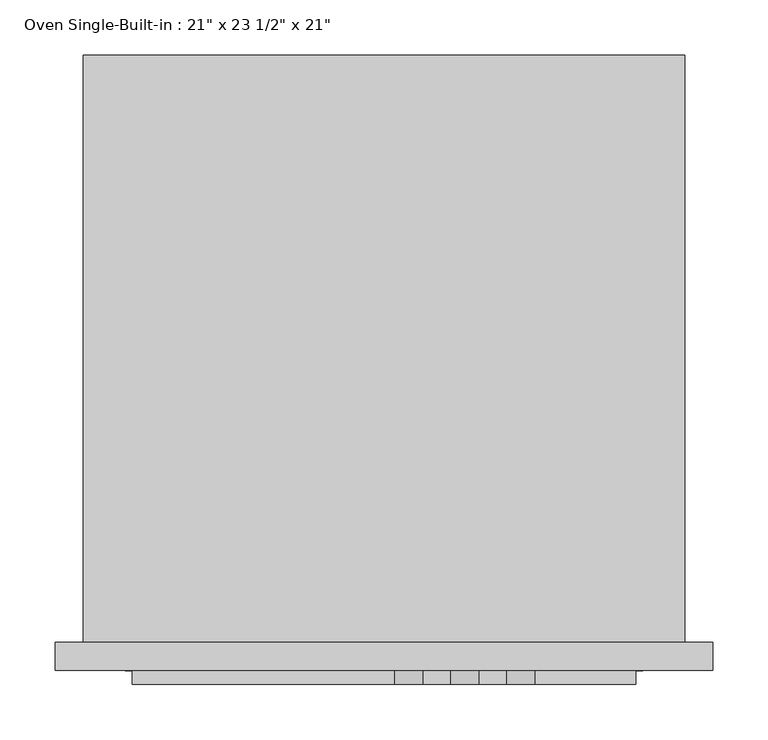
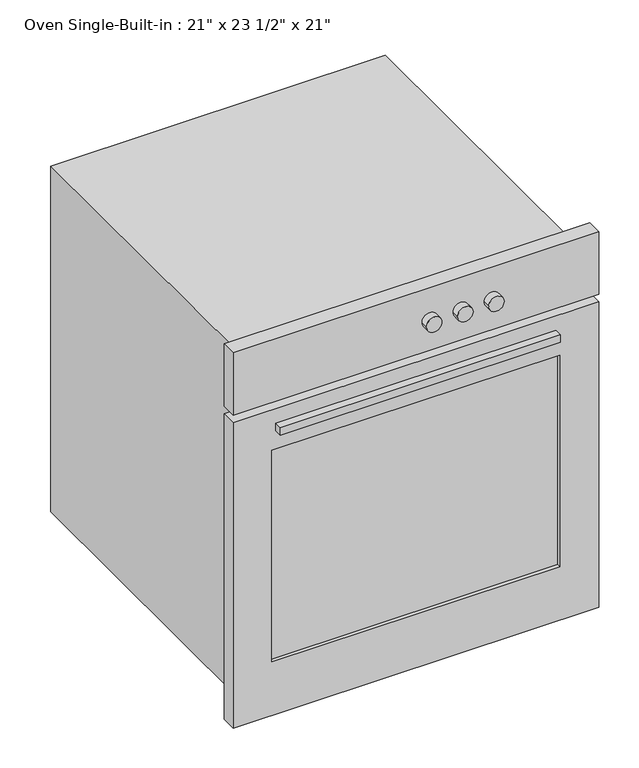
"""IFC4 building model written with IfcOpenShell, lengths in millimetres: proxy geometry."""

from ifc_helpers import new_model, si_unit, point, frame, frame_2d, origin, place, context, project, spatial, polyline, circle_curve, trimmed, segment, composite_curve, outline, extrude, faceted_brep, source, transform, mapped, element, save


def proxy_34c9623a(model_context):
    return source(origin(), model_context, "Body", "SolidModel", [
        faceted_brep([(237.8750727, -125.6341411, 838.2), (-308.2249273, -125.6341411, 838.2), (-308.2249273, -125.6341411, 241.3), (237.8750727, -125.6341411, 241.3), (212.4750727, -125.6341411, 812.8), (212.4750727, -125.6341411, 266.7), (-282.8249273, -125.6341411, 266.7), (-282.8249273, -125.6341411, 812.8), (237.8750727, 407.7658589, 838.2), (237.8750727, 407.7658589, 241.3), (-308.2249273, 407.7658589, 241.3), (-308.2249273, 407.7658589, 838.2), (212.4750727, 382.1090259, 812.8), (212.4750727, 382.1090259, 266.7), (-282.8249273, 382.1090259, 266.7), (-282.8249273, 382.1090259, 812.8)], [[[0, 1, 2, 3], [4, 5, 6, 7]], [[8, 9, 10, 11]], [[1, 0, 8, 11]], [[2, 1, 11, 10]], [[3, 2, 10, 9]], [[0, 3, 9, 8]], [[5, 4, 12, 13]], [[6, 5, 13, 14]], [[7, 6, 14, 15]], [[4, 7, 15, 12]], [[13, 12, 15, 14]]]),
        extrude(outline(polyline([(212.4750727, -125.6341411), (-282.8249273, -125.6341411), (-282.8249273, -100.2341411), (212.4750727, -100.2341411), (212.4750727, -125.6341411)])), frame((0.0, 0.0, 717.6220137), z_axis=(0.0, 0.0, 1.0), x_axis=(1.0, 0.0, 0.0)), (0.0, 0.0, 1.0), 95.1779863),
        extrude(outline(composite_curve([segment(trimmed(circle_curve(frame_2d((807.921693, -12.6998447)), 12.7), [point((807.921693, -25.3998447))], [point((807.921693, 0.0001553))], False, "CARTESIAN"), True, "CONTINUOUS"), segment(trimmed(circle_curve(frame_2d((807.921693, -12.6998447)), 12.7), [point((807.921693, 0.0001553))], [point((807.921693, -25.3998447))], False, "CARTESIAN"), True, "CONTINUOUS")], self_intersect=False)), frame((0.0, -163.7341411, 0.0), z_axis=(0.0, 1.0, 0.0), x_axis=(0.0, 0.0, 1.0)), (0.0, 0.0, 1.0), 12.7),
        extrude(outline(composite_curve([segment(trimmed(circle_curve(frame_2d((807.921693, 38.1001553)), 12.7), [point((807.921693, 25.4001553))], [point((807.921693, 50.8001553))], False, "CARTESIAN"), True, "CONTINUOUS"), segment(trimmed(circle_curve(frame_2d((807.921693, 38.1001553)), 12.7), [point((807.921693, 50.8001553))], [point((807.921693, 25.4001553))], False, "CARTESIAN"), True, "CONTINUOUS")], self_intersect=False)), frame((0.0, -163.7341411, 0.0), z_axis=(0.0, 1.0, 0.0), x_axis=(0.0, 0.0, 1.0)), (0.0, 0.0, 1.0), 12.7),
        extrude(outline(composite_curve([segment(trimmed(circle_curve(frame_2d((807.921693, 88.9001553)), 12.7), [point((807.921693, 76.2001553))], [point((807.921693, 101.6001553))], False, "CARTESIAN"), True, "CONTINUOUS"), segment(trimmed(circle_curve(frame_2d((807.921693, 88.9001553)), 12.7), [point((807.921693, 101.6001553))], [point((807.921693, 76.2001553))], False, "CARTESIAN"), True, "CONTINUOUS")], self_intersect=False)), frame((0.0, -163.7341411, 0.0), z_axis=(0.0, 1.0, 0.0), x_axis=(0.0, 0.0, 1.0)), (0.0, 0.0, 1.0), 12.7),
        extrude(outline(polyline([(193.4250727, -163.7341411), (-263.7749273, -163.7341411), (-263.7749273, -151.0341411), (193.4250727, -151.0341411), (193.4250727, -163.7341411)])), frame((0.0, 0.0, 704.9220137), z_axis=(0.0, 0.0, 1.0), x_axis=(1.0, 0.0, 0.0)), (0.0, 0.0, 1.0), 12.7),
        extrude(outline(polyline([(199.7750727, -144.6841411), (-270.1249273, -144.6841411), (-270.1249273, -138.3341411), (199.7750727, -138.3341411), (199.7750727, -144.6841411)])), frame((0.0, 0.0, 307.975), z_axis=(0.0, 0.0, 1.0), x_axis=(1.0, 0.0, 0.0)), (0.0, 0.0, 1.0), 365.125),
        extrude(outline(polyline([(263.2750727, -151.0341411), (-333.6249273, -151.0341411), (-333.6249273, -125.6341411), (263.2750727, -125.6341411), (263.2750727, -151.0341411)])), frame((0.0, 0.0, 755.65), z_axis=(0.0, 0.0, 1.0), x_axis=(1.0, 0.0, 0.0)), (0.0, 0.0, 1.0), 107.95),
        extrude(outline(polyline([(742.95, 263.2750727), (742.95, -333.6249273), (215.9, -333.6249273), (215.9, 263.2750727), (742.95, 263.2750727)]), holes=[polyline([(673.1, 199.7750727), (307.975, 199.7750727), (307.975, -270.1249273), (673.1, -270.1249273), (673.1, 199.7750727)])]), frame((0.0, -151.0341411, 0.0), z_axis=(0.0, 1.0, 0.0), x_axis=(0.0, 0.0, 1.0)), (0.0, 0.0, 1.0), 25.4),
    ])


if __name__ == "__main__":
    model = new_model("IFC4")
    model_context = context("Model", 3, world=origin())
    ifc_project = project(units=[si_unit("LENGTHUNIT", "METRE", prefix="MILLI")], contexts=[model_context])
    site = spatial("IfcSite", under=ifc_project)
    building = spatial("IfcBuilding", under=site)
    placement = place(None, origin())
    proxy_shape = proxy_34c9623a(model_context)
    element("IfcBuildingElementProxy", 1, Name="Oven Single-Built-in : 21\" x 23 1/2\" x 21\"", ObjectType="Oven Single-Built-in : 21\" x 23 1/2\" x 21\"", at=placement, inside=building, context=model_context, shape_type="MappedRepresentation", body=[
        mapped(proxy_shape, transform((0.0, 0.0, 0.0), x_axis=(1.0, 0.0, 0.0), y_axis=(0.0, 1.0, 0.0), z_axis=(0.0, 0.0, 1.0))),
    ])
    save(model, "model.ifc")

# Revit data of these elements
# Type "Oven Single-Built-in : 21\" x 23 1/2\" x 21\""
#   Label = "OVEN"
#   Assembly Code = "E1090400"
#   Depth = 1' - 9"
#   Height = 1' - 11 1/2"
#   Install Height = 0' - 9 1/2"
#   Width = 1' - 9 1/2"
#   Oven Material = Metal - Stainless Steel, Polished
#   Default Elevation = 0
# Element 1 (IfcBuildingElementProxy, "Oven Single-Built-in : 21\" x 23 1/2\" x 21\"")
#   Materials on its faces: "Steel", "Metal - Stainless Steel, Polished", "Glass"
# Materials
#   "Metal - Stainless Steel, Polished": class "Metal", colour RGB 215 215 215, transparency 0
#   "Steel": class "Metal", colour RGB 247 247 247, transparency 0, Description = "Steel, mill finish", Cost = 0
#   "Glass": class "Glass", colour RGB 0 128 192, transparency 0.75, Description = "Soda Lime Glass", Cost = 0
